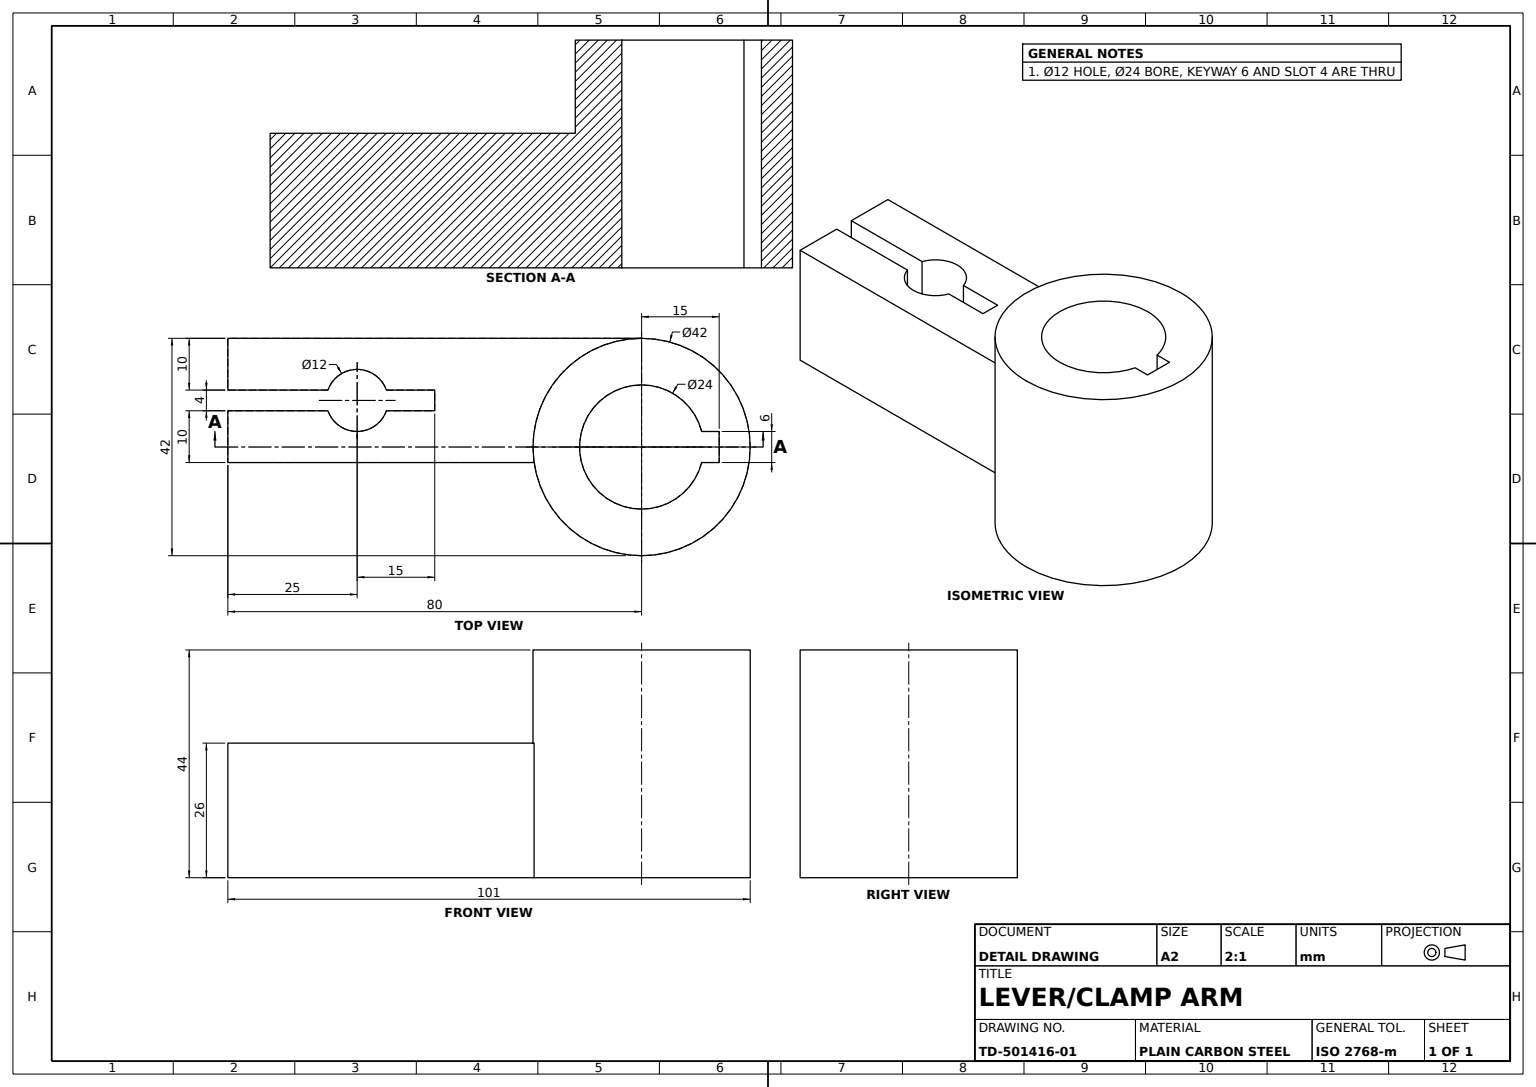
SolidWorks part; units mm, degrees
material "Plain Carbon Steel"
ref_plane "Front Plane" through (0, 0, 0) normal (0, 0, 1) x (1, 0, 0)
ref_plane "Top Plane" through (0, 0, 0) normal (0, 1, 0) x (1, 0, 0)
ref_plane "Right Plane" through (0, 0, 0) normal (1, 0, 0) x (0, 0, -1)
sketch "Lever Arm Profile" plane through (0, 0, 0) normal (0, 0, 1) x (1, 0, 0)
  line L0 (0, 0) -> (80, 0)
  line L1 (0, 0) -> (0, 26)
  line L2 (0, 26) -> (80, 26)
  line L3 (80, 26) -> (80, 0)
  dimension "D1" = 80
  dimension "D2" = 26
extrude "Lever Arm 80x26" add sketch "Lever Arm Profile" against normal blind 24
sketch "Hub Profile Ø42" plane through (0, 26, 0) normal (0, 1, 0) x (1, 0, 0)
  line L1 (80, 24) -> (80, 0) construction
  circle A0 centre (80, 3) radius 21
  dimension "D2" = 42
  dimension "D1" = 21
extrude "Hub Boss Ø42" add sketch "Hub Profile Ø42" against normal blind 26
sketch "Hub Extension Profile Ø42" plane through (0, 26, 0) normal (0, 1, 0) x (1, 0, 0)
  circle A0 centre (80, 3) radius 21
  dimension "D1" = 42
extrude "Hub Extension Ø42" add sketch "Hub Extension Profile Ø42" along normal blind 18
sketch "Clamp Slot Profile" plane through (0, 26, 0) normal (0, 1, 0) x (1, 0, 0)
  line L0 (80, 24) -> (0, 24) construction
  line L1 (0, 24) -> (0, 0) construction
  line L2 (0, 14) -> (0, 10)
  line L3 (0, 14) -> (19.3431, 14)
  line L4 (40, 14) -> (40, 10)
  line L5 (40, 10) -> (30.6569, 10)
  line L6 (30.6569, 14) -> (40, 14)
  line L7 (19.3431, 10) -> (0, 10)
  arc A0 (19.3431, 10) -> (30.6569, 10) centre (25, 12) ccw
  arc A1 (30.6569, 14) -> (19.3431, 14) centre (25, 12) ccw
  dimension "D2" = 12
  dimension "D1" = 10
  dimension "D3" = 11.3137
  dimension "D4" = 40
  dimension "D5" = 4
  dimension "D6" = 19.3431
  dimension "D7" = 4
extrude "Clamp Split Slot" cut sketch "Clamp Slot Profile" against normal blind 30
sketch "Keyed Bore Profile" plane through (0, 44, 0) normal (0, 1, 0) x (1, 0, 0)
  line L2 (95, 6) -> (91.619, 6)
  line L4 (91.619, 0) -> (95, 0)
  line L6 (95, 6) -> (95, 0)
  arc A0 (91.619, 6) -> (91.619, 0) centre (80, 3) ccw
  dimension "D1" = 24
  dimension "D2" = 6
  dimension "D3" = 3.381
  dimension "D4" = 15
  dimension "D5" = 3.381
extrude "Keyed Bore Ø24" cut sketch "Keyed Bore Profile" against normal blind 50
